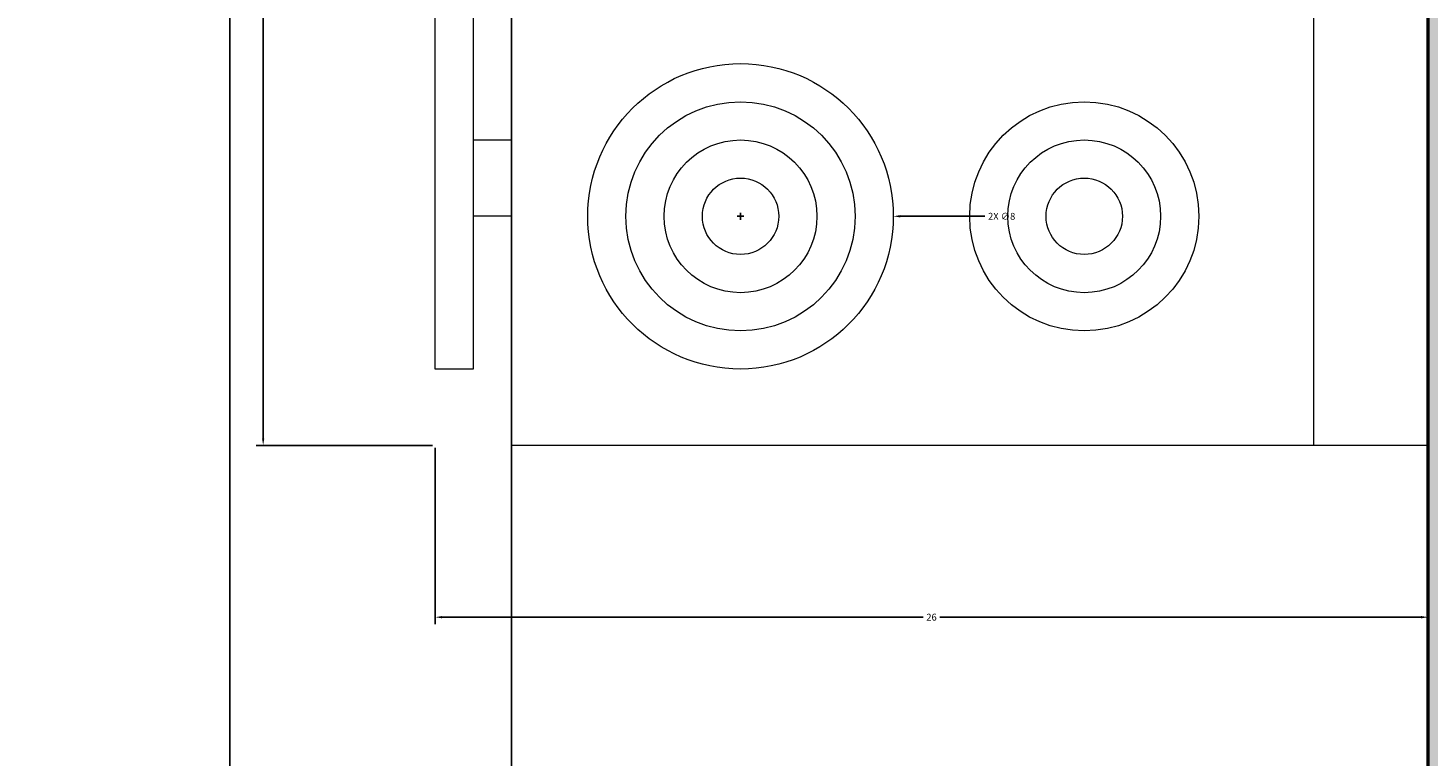
# Model space of a CAD drawing. Units: inches. Extents: x 2231 to 2461, y 2045 to 2455.
# Tile 30 of 95: x 2396 to 2433, y 2112 to 2132. Entities that reach past the tile are written whole.
import ezdxf

# ---------------------------------------------------------------- set-up
doc = ezdxf.new("R2010")
doc.units = ezdxf.units.IN
for name, color, linetype, lineweight in [('A-ANNO-DIMS', 2, 'Continuous', 18), ('A-EQPM', 8, 'Continuous', 18), ('A-FLOR-CASE', 8, 'Continuous', 25), ('A-WALL', 7, 'Continuous', 50)]:
    doc.layers.add(name, color=color, linetype=linetype, lineweight=lineweight)
doc.layers.add('A-WALL-PATT', color=18, linetype='Continuous', lineweight=13, true_color=0x000000)
doc.styles.get("Standard").update_dxf_attribs({"font": 'arial.ttf'})
doc.dimstyles.get("Standard").update_dxf_attribs({"dimtxt": 0.18, "dimasz": 0.18, "dimexe": 0.18, "dimexo": 0.0625, "dimgap": 0.09, "dimtad": 0, "dimtih": 1, "dimtoh": 1, "dimdec": 4, "dimzin": 0, "dimdsep": 46, "dimtxsty": 'Standard', "dimcen": 0.09, "dimadec": 0, "dimazin": 0, "dimtfac": 1, "dimtdec": 4, "dimtofl": 0, "dimtmove": 0, "dimatfit": 3, "dimfxl": 1, "dimtolj": 1, "dimtzin": 0, "dimarcsym": 0})

# ---------------------------------------------------------------- blocks, each defined once
blk = doc.blocks.new('Range-Oven - 30 in top')
for p, q in [((0, -3), (30, -3)), ((12, -6), (18, -6)), ((13, -20), (13, -6)), ((14, -6), (14, -20)), ((15, -20), (15, -6)), ((16, -6), (16, -20)), ((17, -20), (17, -6)), ((18, -20), (12, -20)), ((6, -24), (6, -25)), ((8, -25), (8, -24)), ((22, -25), (22, -24)), ((24, -24), (24, -25))]:
    blk.add_line(p, q)
for points in [[(0, -24), (0, 0), (30, 0), (30, -24)], [(12, -21), (12, -5), (18, -5), (18, -21)], [(2, -26), (2, -25), (28, -25), (28, -26)]]:
    blk.add_lwpolyline(points, close=True)
for centre, radius in [((6, -9), 4), ((6, -9), 3), ((24, -9), 3), ((6, -9), 2), ((24, -9), 2), ((6, -9), 1), ((24, -9), 1), ((24, -18), 4), ((6, -18), 3), ((24, -18), 3), ((6, -18), 2), ((24, -18), 2), ((6, -18), 1), ((24, -18), 1)]:
    blk.add_circle(centre, radius)
blk = doc.blocks.new('*D27')
at = {"layer": 'A-ANNO-DIMS', "color": 0, "lineweight": -2, "transparency": 16777216}
for p, q in [((2406.731, 2150.615), (2402.114, 2150.615)), ((2402.294, 2150.435), (2402.294, 2135.798)), ((2402.294, 2120.795), (2402.294, 2135.431)), ((2406.731, 2120.615), (2402.114, 2120.615))]:
    blk.add_line(p, q, dxfattribs=at)
at = {"layer": 'A-ANNO-DIMS', "color": 0, "transparency": 16777216}
for points in [[(2402.264, 2150.435), (2402.324, 2150.435), (2402.294, 2150.615)], [(2402.264, 2120.795), (2402.324, 2120.795), (2402.294, 2120.615)]]:
    blk.add_solid(points, dxfattribs=at)
at = {"layer": 'Defpoints', "color": 0, "transparency": 16777216}
for p in [(2406.794, 2150.615), (2402.294, 2120.615), (2406.794, 2120.615)]:
    blk.add_point(p, dxfattribs=at)
at = {"layer": 'A-ANNO-DIMS', "color": 0, "transparency": 16777216, "insert": (2402.294, 2135.615), "char_height": 0.18, "attachment_point": 5}
blk.add_mtext('\\A1;RANGE 30', dxfattribs=at)
blk = doc.blocks.new('*D28')
at = {"layer": 'A-ANNO-DIMS', "color": 0, "lineweight": -2, "transparency": 16777216}
for p, q in [((2406.794, 2120.552), (2406.794, 2115.935)), ((2432.794, 2120.552), (2432.794, 2115.935)), ((2406.974, 2116.115), (2419.573, 2116.115)), ((2432.614, 2116.115), (2420.014, 2116.115))]:
    blk.add_line(p, q, dxfattribs=at)
at = {"layer": 'A-ANNO-DIMS', "color": 0, "transparency": 16777216}
for points in [[(2406.974, 2116.145), (2406.974, 2116.085), (2406.794, 2116.115)], [(2432.614, 2116.145), (2432.614, 2116.085), (2432.794, 2116.115)]]:
    blk.add_solid(points, dxfattribs=at)
at = {"layer": 'Defpoints', "color": 0, "transparency": 16777216}
for p in [(2406.794, 2120.615), (2432.794, 2120.615), (2432.794, 2116.115)]:
    blk.add_point(p, dxfattribs=at)
at = {"layer": 'A-ANNO-DIMS', "color": 0, "transparency": 16777216, "insert": (2419.794, 2116.115), "char_height": 0.18, "attachment_point": 5}
blk.add_mtext('\\A1;26', dxfattribs=at)
blk = doc.blocks.new('*D66')
at = {"layer": 'A-ANNO-DIMS', "color": 0, "lineweight": -2, "transparency": 16777216}
for p, q in [((2348.189, 2096.895), (2348.189, 2454.645)), ((2408.794, 2096.895), (2408.794, 2454.645)), ((2348.369, 2454.465), (2378.167, 2454.465)), ((2408.614, 2454.465), (2378.815, 2454.465))]:
    blk.add_line(p, q, dxfattribs=at)
at = {"layer": 'A-ANNO-DIMS', "color": 0, "transparency": 16777216}
for points in [[(2348.369, 2454.495), (2348.369, 2454.435), (2348.189, 2454.465)], [(2408.614, 2454.495), (2408.614, 2454.435), (2408.794, 2454.465)]]:
    blk.add_solid(points, dxfattribs=at)
at = {"layer": 'Defpoints', "color": 0, "transparency": 16777216}
for p in [(2408.794, 2454.465), (2348.189, 2096.833), (2408.794, 2096.833)]:
    blk.add_point(p, dxfattribs=at)
at = {"layer": 'A-ANNO-DIMS', "color": 0, "transparency": 16777216, "insert": (2378.491, 2454.465), "char_height": 0.18, "attachment_point": 5}
blk.add_mtext('\\A1;60.6', dxfattribs=at)
blk = doc.blocks.new('*D71')
at = {"layer": 'A-ANNO-DIMS', "color": 0, "lineweight": -2, "transparency": 16777216}
for p, q in [((2401.422, 2092.979), (2401.422, 2454.645)), ((2408.794, 2096.895), (2408.794, 2454.645)), ((2401.602, 2454.465), (2404.732, 2454.465)), ((2408.614, 2454.465), (2405.483, 2454.465))]:
    blk.add_line(p, q, dxfattribs=at)
at = {"layer": 'A-ANNO-DIMS', "color": 0, "transparency": 16777216}
for points in [[(2401.602, 2454.495), (2401.602, 2454.435), (2401.422, 2454.465)], [(2408.614, 2454.495), (2408.614, 2454.435), (2408.794, 2454.465)]]:
    blk.add_solid(points, dxfattribs=at)
at = {"layer": 'Defpoints', "color": 0, "transparency": 16777216}
for p in [(2408.794, 2454.465), (2408.794, 2096.833), (2401.422, 2092.917)]:
    blk.add_point(p, dxfattribs=at)
at = {"layer": 'A-ANNO-DIMS', "color": 0, "transparency": 16777216, "insert": (2405.108, 2454.465), "char_height": 0.18, "attachment_point": 5}
blk.add_mtext('\\A1;7.371', dxfattribs=at)
blk = doc.blocks.new('*D78')
at = {"layer": 'A-ANNO-DIMS', "color": 0, "lineweight": -2, "transparency": 16777216}
for p, q in [((2414.704, 2126.615), (2414.884, 2126.615)), ((2414.794, 2126.525), (2414.794, 2126.705)), ((2421.194, 2126.615), (2418.974, 2126.615))]:
    blk.add_line(p, q, dxfattribs=at)
at = {"layer": 'A-ANNO-DIMS', "color": 0, "transparency": 16777216}
blk.add_solid([(2418.974, 2126.645), (2418.974, 2126.585), (2418.794, 2126.615)], dxfattribs=at)
at = {"layer": 'Defpoints', "color": 0, "transparency": 16777216}
for p in [(2410.794, 2126.614), (2418.794, 2126.615)]:
    blk.add_point(p, dxfattribs=at)
at = {"layer": 'A-ANNO-DIMS', "color": 0, "transparency": 16777216, "insert": (2421.631, 2126.615), "char_height": 0.18, "attachment_point": 5}
blk.add_mtext('\\A1;2X ∅8', dxfattribs=at)

msp = doc.modelspace()

# ---------------------------------------------------------------- hatches: boundary and pattern name
at = {"layer": 'A-WALL-PATT'}
h = msp.add_hatch(color=256, dxfattribs=at)
h.dxf.hatch_style = 1
h.paths.add_polyline_path([(2441.7935, 2269.1535), (2432.7935, 2269.1535), (2432.7935, 2186.8328), (2396.7935, 2186.8328), (2396.7935, 2286.8328), (2394.7935, 2286.8328), (2394.7935, 2186.8328), (2334.7935, 2186.8328), (2334.7935, 2182.8328), (2432.7935, 2182.8328), (2432.7935, 2072.8328), (2416.6639, 2072.8328), (2416.6639, 2063.8328), (2441.7935, 2063.8328)])
h.paths.add_polyline_path([(2368.6639, 2072.8328), (2367.04, 2072.8328), (2330.7942, 2072.8328), (2330.7397, 2063.8328), (2368.6639, 2063.8328)])
h.paths.add_polyline_path([(2300.7392, 2068.3328), (2300.7392, 2072.8328), (2298.7935, 2072.8328), (2294.7935, 2072.8328), (2258.7935, 2072.8328), (2258.7935, 2120.8328), (2294.7935, 2120.8328), (2298.7935, 2120.8328), (2298.7935, 2128.8328), (2294.7935, 2128.8328), (2294.7935, 2124.8328), (2258.7935, 2124.8328), (2258.7935, 2182.8328), (2294.7935, 2182.8328), (2294.7935, 2174.8328), (2298.7935, 2174.8328), (2298.7935, 2182.8328), (2304.7935, 2182.8328), (2304.7935, 2186.8328), (2258.7935, 2186.8328), (2258.7935, 2221.999), (2249.7935, 2221.999), (2249.7935, 2063.8328), (2300.7392, 2063.8328)])
h.paths.add_polyline_path([(2391.9338, 2435.8328), (2333.82, 2435.8328), (2333.82, 2426.8328), (2368.7935, 2426.8328), (2368.7935, 2374.9508), (2368.7935, 2370.8328), (2372.3935, 2370.8328), (2372.7935, 2370.8328), (2372.7935, 2426.8328), (2391.9338, 2426.8328)])
h.paths.add_polyline_path([(2441.7935, 2435.8328), (2415.9338, 2435.8328), (2415.9338, 2426.8328), (2432.7935, 2426.8328), (2432.7935, 2334.8328), (2372.7935, 2334.8328), (2372.7935, 2346.8328), (2368.7935, 2346.8328), (2368.7935, 2306.8328), (2360.7935, 2306.8328), (2360.7935, 2302.8328), (2368.7935, 2302.8328), (2372.7935, 2302.8328), (2372.7935, 2330.8328), (2432.7935, 2330.8328), (2432.7935, 2317.1535), (2441.7935, 2317.1535)])
h.paths.add_polyline_path([(2285.82, 2435.8328), (2249.7935, 2435.8328), (2249.7935, 2269.999), (2258.7935, 2269.999), (2258.7935, 2302.8328), (2318.8168, 2302.8328), (2330.7935, 2302.8328), (2330.7935, 2306.8328), (2258.7935, 2306.8328), (2258.7935, 2426.8328), (2285.82, 2426.8328)])

# ---------------------------------------------------------------- linework, layer by layer
at = {"layer": 'A-FLOR-CASE'}
msp.add_line((2408.7935, 2182.8328), (2408.7935, 2096.8328), dxfattribs=at)
at = {"layer": 'A-WALL'}
msp.add_line((2432.7935, 2182.8328), (2432.7935, 2072.8328), dxfattribs=at)

# ---------------------------------------------------------------- block references
at = {"layer": 'A-EQPM', "rotation": 270}
msp.add_blockref('Range-Oven - 30 in top', (2432.7935, 2150.6145), dxfattribs=at)

# ---------------------------------------------------------------- dimensions: what is measured, and where the dimension line sits
at = {"layer": 'A-ANNO-DIMS'}
for base, p1, p2, override, picture, middle in [((2408.7935, 2454.4653), (2348.1888, 2096.8328), (2408.7935, 2096.8328), {"dimdec": 1, "dimlfac": 1, "dimrnd": 0, "dimzin": 0, "dimdsep": 46, "dimlunit": 2}, '*D66', (2378.4912, 2454.4653)), ((2408.7935, 2454.4653), (2401.4221, 2092.9167), (2408.7935, 2096.8328), {"dimdec": 3, "dimlfac": 1, "dimrnd": 0, "dimzin": 0, "dimdsep": 46, "dimlunit": 2}, '*D71', (2405.1078, 2454.4653)), ((2432.7935, 2116.1145), (2406.7935, 2120.6145), (2432.7935, 2120.6145), {"dimdec": 0, "dimlfac": 1, "dimrnd": 0, "dimzin": 0, "dimdsep": 46, "dimlunit": 2}, '*D28', (2419.7935, 2116.1145))]:
    dim = msp.add_linear_dim(base=base, p1=p1, p2=p2, dimstyle='Standard', override=override, dxfattribs=at)
    dim.commit()
    dim.dimension.update_dxf_attribs({"geometry": picture, "text_midpoint": middle})
dim = msp.add_linear_dim(base=(2402.2935, 2120.6145), p1=(2406.7935, 2150.6145), p2=(2406.7935, 2120.6145), angle=270, text='RANGE <>', dimstyle='Standard', override={"dimdec": 0, "dimlfac": 1, "dimrnd": 0, "dimzin": 0, "dimdsep": 46, "dimlunit": 2}, dxfattribs=at)
dim.commit()
dim.dimension.update_dxf_attribs({"geometry": '*D27', "text_midpoint": (2402.2935, 2135.6145)})
dim = msp.add_diameter_dim_2p(p1=(2410.7935, 2126.6141), p2=(2418.7935, 2126.615), text='2X <>', dimstyle='Standard', override={"dimdec": 0, "dimlfac": 1, "dimrnd": 0, "dimzin": 0, "dimdsep": 46, "dimlunit": 2}, dxfattribs=at)
dim.commit()
dim.dimension.update_dxf_attribs({"geometry": '*D78', "text_midpoint": (2421.1935, 2126.6153), "dimtype": 163})

doc.saveas('drawing.dxf')
